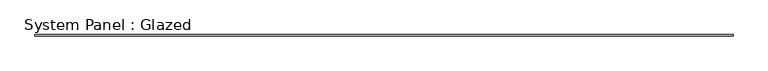
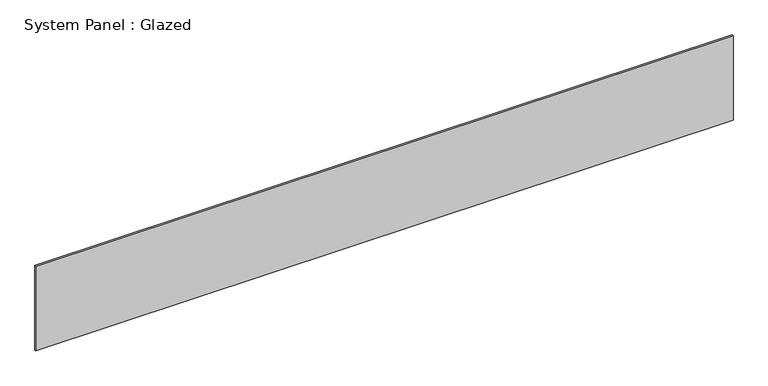
"""IFC4 building model written with IfcOpenShell, lengths in millimetres: plate geometry, System Panel : Glazed."""

from ifc_helpers import new_model, si_unit, origin, origin_with_axes, place, context, project, spatial, polyline, outline, extrude, source, transform, mapped, element, save


def system_panel_glazed_372aa133(model_context):
    return source(origin(), model_context, "Body", "SweptSolid", [
        extrude(outline(polyline([(6877.8643402, 19.05), (-6877.8643402, 19.05), (-6877.8643402, 44.45), (6877.8643402, 44.45), (6877.8643402, 19.05)])), origin_with_axes(), (0.0, 0.0, 1.0), 1765.3),
    ])


if __name__ == "__main__":
    model = new_model("IFC4")
    model_context = context("Model", 3, world=origin())
    ifc_project = project(units=[si_unit("LENGTHUNIT", "METRE", prefix="MILLI")], contexts=[model_context])
    site = spatial("IfcSite", under=ifc_project)
    building = spatial("IfcBuilding", under=site)
    placement = place(None, origin())
    system_panel_glazed_shape = system_panel_glazed_372aa133(model_context)
    element("IfcPlate", 1, ObjectType="System Panel : Glazed", at=placement, inside=building, context=model_context, shape_type="MappedRepresentation", body=[
        mapped(system_panel_glazed_shape, transform((0.0, 0.0, 0.0), x_axis=(1.0, 0.0, 0.0), y_axis=(0.0, 1.0, 0.0), z_axis=(0.0, 0.0, 1.0))),
    ])
    save(model, "model.ifc")

# Revit data of these elements
# Type "System Panel : Glazed"
#   Construction Type Id = "GSP4R"
#   Analytic Construction = "1/8 in Pilkington single glazing"
#   Visual Light Transmittance = 0.9
#   Solar Heat Gain Coefficient = 0.86
#   Heat Transfer Coefficient (U) = 1.18115 BTU/(h·ft²·°F)
# Element 1 (IfcPlate, "System Panel : Glazed")
#   Materials on its faces: "Glass"
# Materials
#   "Glass": class "Glass", colour RGB 0 128 192, transparency 0.75, Description = "Soda Lime Glass", Cost = 0
